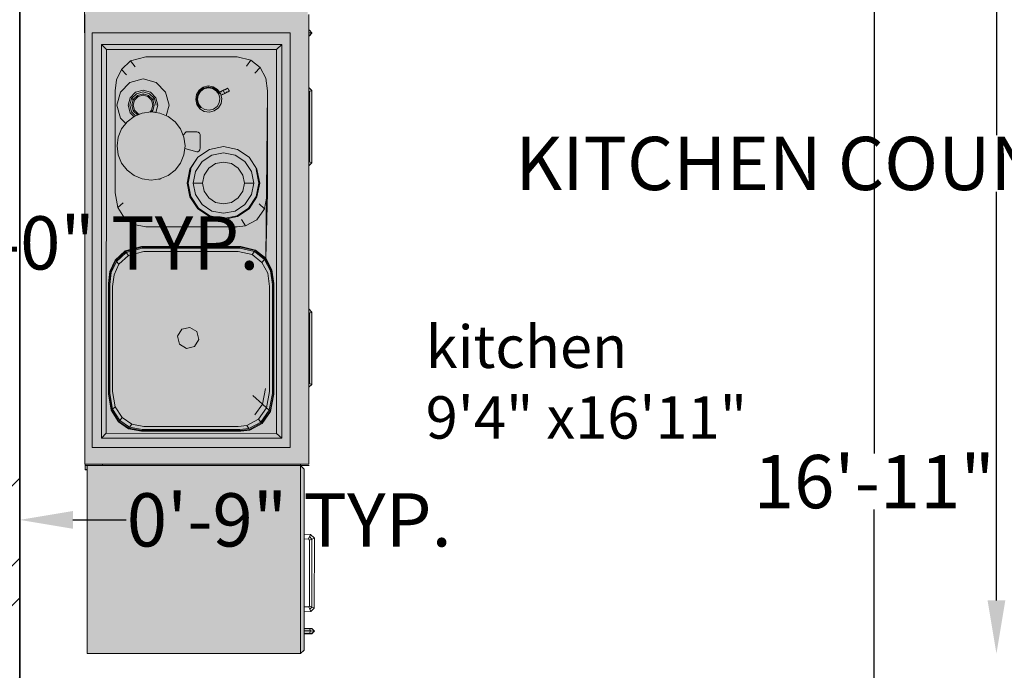
# Model space of a CAD drawing. Units: inches. Extents: x 3614 to 4242, y 2406 to 3033.
# Tile 4 of 10: x 3697 to 3808, y 2823 to 2896. Entities that reach past the tile are written whole.
import ezdxf

# ---------------------------------------------------------------- set-up
doc = ezdxf.new("R2010")
doc.units = ezdxf.units.IN
for name, color, linetype, lineweight in [('A-ANNO-DIMS', 2, 'Continuous', 18), ('A-AREA-IDEN', 7, 'Continuous', 25), ('A-FLOR-FIXT', 9, 'Continuous', 18), ('A-WALL', 7, 'Continuous', 35), ('A-WALL-PATT', 252, 'Continuous', 13)]:
    doc.layers.add(name, color=color, linetype=linetype, lineweight=lineweight)
doc.layers.add('hatch', color=254, linetype='Continuous')
doc.styles.get("Standard").update_dxf_attribs({"font": 'arial.ttf'})
doc.dimstyles.get("Standard").update_dxf_attribs({"dimtxt": 6, "dimasz": 6, "dimexe": 0.18, "dimexo": 0.0625, "dimgap": 0.09, "dimtad": 0, "dimtih": 1, "dimtoh": 1, "dimdec": 4, "dimzin": 0, "dimdsep": 46, "dimlunit": 4, "dimtxsty": 'Standard', "dimcen": 0.09, "dimse1": 1, "dimse2": 1, "dimadec": 0, "dimazin": 0, "dimtfac": 1, "dimtdec": 4, "dimtofl": 0, "dimtmove": 0, "dimatfit": 3, "dimfxl": 1, "dimtolj": 1, "dimtzin": 0, "dimarcsym": 0})

# ---------------------------------------------------------------- blocks, each defined once
blk = doc.blocks.new('kithen1')
at = {"layer": 'hatch'}
blk.add_hatch(color=256, dxfattribs=at).paths.add_polyline_path([(-2799.7, -8.3), (-2273.3, -8.3), (-2273.3, -1.7), (-2257.5, -1.7), (-2257.5, -1.1), (-1023.7, -1.1), (-1023.7, 0), (0, 0), (0, -0.3), (0.3, -0.3), (0.3, -1009.9), (-6.1, -1009.9), (-6.1, -2189.3), (-615.8, -2189.3), (-626.5, -2178.9), (-626.5, -1578.2), (-615.8, -1567.8), (-649.5, -1567.8), (-649.5, -1399.1), (-650.3, -1399.1), (-650.3, -1376.8), (-657.9, -1368.5), (-657.8, -1162.4), (-650.3, -1155.1), (-650.3, -1126.4), (-649.5, -1126.4), (-649.5, -1081.1), (-650.3, -1081.1), (-650.3, -1021.1), (-649.5, -1021.1), (-649.5, -959.1), (-651, -959.1), (-650.7, -903), (-653.5, -903), (-660.6, -895.5), (-660.5, -894.6), (-653.5, -887.1), (-651, -887.1), (-651, -638.7), (-651.2, -638.5), (-898.3, -638.5), (-898.3, -640.4), (-905.9, -647.4), (-906.8, -647.4), (-914.3, -640.4), (-914.3, -638.5), (-971.4, -638.5), (-971.4, -642.6), (-1016.2, -642.6), (-1016.2, -643.9), (-1023.8, -650.9), (-1024.7, -650.9), (-1032.2, -643.9), (-1032.2, -642.6), (-1179.7, -642.6), (-1188.8, -650.9), (-1395.6, -650.9), (-1403.7, -642.6), (-1813.5, -642.6), (-1822.6, -650.9), (-2029.4, -650.9), (-2037.5, -642.6), (-2257.5, -642.6), (-2257.5, -618.1), (-2261.3, -618.1), (-2271.7, -628.7), (-2458, -628.7), (-2727.7, -628.7), (-2727.7, -651.1), (-2735, -658.1), (-2735.9, -658), (-2743.2, -651.1), (-2743.2, -628.7), (-2789.4, -628.7), (-2799.7, -618.1)])
at = {"color": 0}
for p, q in [((0, 0), (-1023.7, 0)), ((-2261.3, -8.3), (-2799.7, -8.3)), ((-2799.7, -8.3), (-2799.7, -618.1)), ((-2273.3, -1.9), (-2273.9, -1.9)), ((-2273.9, -1.9), (-2273.9, -8.3)), ((-2261.3, -1.7), (-2273.3, -1.7)), ((-2273.3, -1.7), (-2273.3, -8.3)), ((-2261.3, -601.6), (-2261.3, -1.7)), ((-2261.3, -618.1), (-2261.3, -8.3)), ((-2261, -8.5), (-2261.3, -8.5)), ((-971.4, -1.1), (-2257.5, -1.1)), ((-2257.5, -1.1), (-2257.5, -642.6)), ((-1023.7, -22.5), (-2210.1, -22.5)), ((-2210.1, -22.5), (-2210.1, -589.1)), ((-1023.7, -589.1), (-1023.7, -22.5)), ((-2257.5, -51.5), (-2261.3, -51.5)), ((-2261.3, -51.5), (-2261.3, -536.3)), ((-2183.7, -48.8), (-1056.9, -48.9)), ((-2169.4, -62.7), (-2183.7, -48.8)), ((-2183.7, -48.8), (-2183.7, -565)), ((-1056.9, -48.9), (-1071, -63.6)), ((-1056.9, -48.9), (-1056.9, -565)), ((-2169.7, -550.2), (-2169.4, -62.7)), ((-1071, -63.6), (-2169.4, -62.7)), ((-2103.6, -76.6), (-2136.6, -97.6)), ((-2135.1, -98.9), (-2102.3, -78.1)), ((-2100.1, -80.6), (-2132.5, -101.2)), ((-2057.7, -68.5), (-2103.6, -76.6)), ((-2102.3, -78.1), (-2056.8, -70)), ((-2100.1, -80.6), (-2102.3, -78.1)), ((-2055, -72.6), (-2100.1, -80.6)), ((-2093.2, -88.3), (-2100.1, -80.6)), ((-2049.7, -80.6), (-2093.2, -88.3)), ((-1740.9, -68.5), (-2057.7, -68.5)), ((-2056.8, -70), (-1741.9, -70)), ((-1743.7, -72.6), (-2055, -72.6)), ((-1749, -80.6), (-2049.7, -80.6)), ((-1716.2, -84.8), (-1749, -80.6)), ((-1709.7, -76.9), (-1743.7, -72.6)), ((-1741.9, -70), (-1707.6, -74.4)), ((-1706.4, -72.9), (-1740.9, -68.5)), ((-1678, -91.5), (-1709.7, -76.9)), ((-1707.6, -74.4), (-1675.5, -89.1)), ((-1674.1, -87.7), (-1706.4, -72.9)), ((-1071, -550.2), (-1071, -63.6)), ((-2136.6, -97.6), (-2156.1, -126.2)), ((-2154.5, -127.3), (-2135.1, -98.9)), ((-2132.5, -101.2), (-2151.7, -129.3)), ((-2124.5, -108.2), (-2143, -135.3)), ((-2132.5, -101.2), (-2135.1, -98.9)), ((-2124.5, -108.2), (-2132.5, -101.2)), ((-2093.2, -88.3), (-2124.5, -108.2)), ((-1685.6, -98.8), (-1716.2, -84.8)), ((-1678, -91.5), (-1685.6, -98.8)), ((-1685.6, -98.8), (-1660.4, -125.8)), ((-1651.9, -119.5), (-1678, -91.5)), ((-1675.5, -89.1), (-1649.1, -117.4)), ((-1647.6, -116.2), (-1674.1, -87.7)), ((-1523.7, -95.6), (-1554, -114.9)), ((-1481.5, -88.1), (-1523.7, -95.6)), ((-1523.7, -95.6), (-1509.8, -111.1)), ((-1189.8, -88.1), (-1481.5, -88.1)), ((-1416.2, -122.1), (-1396, -106.6)), ((-1396, -106.6), (-1372.5, -96.9)), ((-1372.5, -96.9), (-1347.3, -93.6)), ((-1347.3, -93.6), (-1322, -96.9)), ((-1322, -96.9), (-1298.5, -106.6)), ((-1298.5, -106.6), (-1278.3, -122.1)), ((-1283.4, -118.2), (-1268.1, -102.9)), ((-1268.1, -102.9), (-1230.5, -92.9)), ((-1230.5, -92.9), (-1193, -102.9)), ((-1193, -102.9), (-1165.5, -130.3)), ((-1157.9, -92.2), (-1189.8, -88.1)), ((-1128.2, -105.8), (-1157.9, -92.2)), ((-1143.5, -120.5), (-1128.2, -105.8)), ((-1128.2, -105.8), (-1103.8, -132)), ((-2156.1, -126.2), (-2163.3, -163.2)), ((-2161.7, -164.1), (-2154.5, -127.3)), ((-2151.7, -129.3), (-2158.8, -165.7)), ((-2151.7, -129.3), (-2154.5, -127.3)), ((-2143, -135.3), (-2151.7, -129.3)), ((-2149.9, -170.5), (-2143, -135.3)), ((-1660.4, -125.8), (-1651.9, -119.5)), ((-1648.8, -170.4), (-1660.4, -125.8)), ((-1649.1, -117.4), (-1651.9, -119.5)), ((-1651.9, -119.5), (-1639.9, -165.7)), ((-1649.1, -117.4), (-1637, -164.1)), ((-1635.3, -163.2), (-1647.6, -116.2)), ((-1554, -114.9), (-1572, -141.2)), ((-1431.7, -142.2), (-1416.2, -122.1)), ((-1278.3, -122.1), (-1262.8, -142.2)), ((-1252, -130.7), (-1263.1, -141.8)), ((-1249.5, -134.9), (-1261, -146.4)), ((-1246.6, -139.9), (-1258.4, -151.7)), ((-1252, -130.7), (-1230.5, -124.9)), ((-1249.5, -134.9), (-1230.5, -129.8)), ((-1230.5, -135.6), (-1246.6, -139.9)), ((-1246.6, -139.9), (-1244.8, -143)), ((-1244.8, -143), (-1230.5, -139.2)), ((-1230.5, -124.9), (-1209.1, -130.7)), ((-1230.5, -129.8), (-1211.6, -134.9)), ((-1214.5, -139.9), (-1230.5, -135.6)), ((-1230.5, -135.6), (-1230.5, -139.2)), ((-1230.5, -139.2), (-1216.3, -143)), ((-1216.3, -143), (-1214.5, -139.9)), ((-1211.6, -134.9), (-1214.5, -139.9)), ((-1214.5, -139.9), (-1202.7, -151.7)), ((-1211.6, -134.9), (-1197.7, -148.8)), ((-1209.1, -130.7), (-1193.4, -146.3)), ((-1165.5, -130.3), (-1155.5, -167.7)), ((-1103.8, -132), (-1120.8, -144.8)), ((-1103.8, -132), (-1092.5, -175.3)), ((-2163.3, -163.2), (-2163.3, -447.5)), ((-2161.7, -446.6), (-2161.7, -164.1)), ((-2158.8, -165.7), (-2158.8, -445)), ((-1639.9, -165.7), (-1639.9, -445)), ((-1637, -164.1), (-1637, -446.6)), ((-1635.3, -447.4), (-1635.3, -163.2)), ((-1572, -141.2), (-1578.6, -175.3)), ((-1572, -141.2), (-1554.6, -153.3)), ((-1444.8, -190.8), (-1441.5, -165.7)), ((-1441.5, -165.7), (-1431.7, -142.2)), ((-1262.8, -142.2), (-1253, -165.7)), ((-1258.4, -151.7), (-1258.6, -152.3)), ((-1255.2, -153.5), (-1258.4, -151.7)), ((-1255.2, -153.5), (-1256.4, -157.6)), ((-1244.8, -143), (-1255.2, -153.5)), ((-1253, -165.7), (-1249.7, -190.8)), ((-1205.8, -153.5), (-1216.3, -143)), ((-1202.7, -151.7), (-1205.8, -153.5)), ((-1205.8, -153.5), (-1202, -167.7)), ((-1202, -167.7), (-1205.8, -181.9)), ((-1198.4, -167.7), (-1202.7, -151.7)), ((-1202.7, -183.7), (-1198.4, -167.7)), ((-1202, -167.7), (-1198.4, -167.7)), ((-1197.7, -148.8), (-1192.6, -167.7)), ((-1192.6, -167.7), (-1197.7, -186.6)), ((-1193.4, -146.3), (-1187.6, -167.7)), ((-1187.6, -167.7), (-1193.4, -189.1)), ((-1155.5, -167.7), (-1165.5, -205.1)), ((-2149.9, -440.2), (-2149.9, -170.5)), ((-1648.8, -440.2), (-1648.8, -170.4)), ((-1578.6, -175.3), (-1578.6, -437)), ((-1441.5, -216), (-1444.8, -190.8)), ((-1249.7, -190.8), (-1253, -216)), ((-1250.2, -186.9), (-1244.8, -192.3)), ((-1246.6, -195.5), (-1249.9, -192.2)), ((-1244.8, -192.3), (-1246.6, -195.5)), ((-1230.5, -199.7), (-1246.6, -195.5)), ((-1230.5, -196.1), (-1244.8, -192.3)), ((-1216.3, -192.3), (-1230.5, -196.1)), ((-1214.5, -195.5), (-1230.5, -199.7)), ((-1230.5, -196.1), (-1230.5, -199.7)), ((-1205.8, -181.9), (-1216.3, -192.3)), ((-1216.3, -192.3), (-1214.5, -195.5)), ((-1214.5, -195.5), (-1202.7, -183.7)), ((-1211.6, -200.5), (-1214.5, -195.5)), ((-1197.7, -186.6), (-1211.6, -200.5)), ((-1193.4, -189.1), (-1209.1, -204.7)), ((-1205.8, -181.9), (-1202.7, -183.7)), ((-1092.5, -175.3), (-1092.5, -437)), ((-1442, -212), (-1442.1, -213.6)), ((-1442.1, -213.6), (-1441.9, -216.3)), ((-1441.9, -216.3), (-1441.5, -218.2)), ((-1431.7, -239.4), (-1441.5, -216)), ((-1441.5, -218.2), (-1440.8, -218.9)), ((-1440.8, -218.9), (-1440.3, -218.9)), ((-1253, -216), (-1262.8, -239.4)), ((-1230.5, -210.4), (-1251.6, -204.8)), ((-1250.8, -199.1), (-1249.5, -200.5)), ((-1211.6, -200.5), (-1230.5, -205.5)), ((-1209.1, -204.7), (-1230.5, -210.4)), ((-1165.5, -205.1), (-1193, -232.5)), ((-1416.2, -259.6), (-1431.7, -239.4)), ((-1262.8, -239.4), (-1278.3, -259.6)), ((-1230.5, -242.5), (-1260.7, -234.4)), ((-1193, -232.5), (-1230.5, -242.5)), ((-1914.6, -272.1), (-1926.9, -292)), ((-1891.8, -266.6), (-1914.6, -272.1)), ((-1871.8, -278.8), (-1891.8, -266.6)), ((-1866.3, -301.6), (-1871.8, -278.8)), ((-1396, -275), (-1416.2, -259.6)), ((-1372.5, -284.8), (-1396, -275)), ((-1298.5, -275), (-1322, -284.8)), ((-1278.3, -259.6), (-1298.5, -275)), ((-1926.9, -292), (-1921.4, -314.8)), ((-1878.5, -321.5), (-1866.3, -301.6)), ((-1526.8, -324.6), (-1493.1, -302.1)), ((-1493.1, -302.2), (-1526.8, -324.6)), ((-1492.2, -304.2), (-1525.2, -326.2)), ((-1493.1, -302.1), (-1453.2, -294.2)), ((-1453.2, -294.3), (-1493.1, -302.2)), ((-1453.2, -296.5), (-1492.2, -304.2)), ((-1453.2, -294.2), (-1413.4, -302.1)), ((-1413.4, -302.2), (-1453.2, -294.3)), ((-1453.2, -294.3), (-1453.2, -296.5)), ((-1453.2, -296.5), (-1414.2, -304.2)), ((-1413.4, -302.1), (-1379.6, -324.6)), ((-1379.6, -324.6), (-1413.4, -302.2)), ((-1347.3, -288.1), (-1372.5, -284.8)), ((-1364, -321.4), (-1354.5, -287.1)), ((-1322, -284.8), (-1347.3, -288.1)), ((-1316.5, -282.5), (-1307.2, -290.8)), ((-1307.2, -290.8), (-1307.2, -321.4)), ((-1921.4, -314.8), (-1901.4, -327)), ((-1901.4, -327), (-1878.5, -321.5)), ((-1526.8, -324.6), (-1549.4, -358.3)), ((-1549.4, -358.3), (-1526.8, -324.6)), ((-1525.2, -326.2), (-1547.3, -359.2)), ((-1514.5, -337), (-1533.3, -365)), ((-1486.4, -318.2), (-1514.5, -337)), ((-1453.2, -311.7), (-1486.4, -318.2)), ((-1453.2, -311.7), (-1420.1, -318.2)), ((-1453.2, -338.2), (-1453.2, -311.7)), ((-1420.1, -318.2), (-1392, -337)), ((-1392, -337), (-1373.2, -365)), ((-1379.6, -324.6), (-1357, -358.3)), ((-1357, -358.3), (-1379.6, -324.6)), ((-1363.6, -324.3), (-1364, -321.4)), ((-1361.6, -328), (-1363.6, -324.3)), ((-1357.9, -330.6), (-1361.6, -328)), ((-1352.7, -331.6), (-1357.9, -330.6)), ((-1318.5, -331.6), (-1352.7, -331.6)), ((-1314.3, -331), (-1318.5, -331.6)), ((-1310.7, -329.1), (-1314.3, -331)), ((-1308.2, -326), (-1310.7, -329.1)), ((-1307.2, -321.4), (-1308.2, -326)), ((-1248.3, -343.1), (-1240.7, -330.6)), ((-1243.2, -344.9), (-1236.8, -334.2)), ((-1240.7, -330.6), (-1228.9, -321.9)), ((-1227.6, -324.8), (-1238.3, -332.8)), ((-1236.8, -334.2), (-1226.7, -326.8)), ((-1228.9, -321.9), (-1214.7, -318.4)), ((-1227.6, -324.8), (-1228.3, -323.3)), ((-1214.6, -321.6), (-1227.6, -324.8)), ((-1226.7, -326.8), (-1214.5, -323.7)), ((-1214.7, -318.4), (-1200.3, -320.6)), ((-1214.7, -319.9), (-1214.6, -321.6)), ((-1214.6, -321.6), (-1201.4, -323.6)), ((-1214.5, -323.7), (-1202.1, -325.6)), ((-1202.1, -325.6), (-1191.3, -332)), ((-1201.4, -323.6), (-1200.8, -322)), ((-1201.4, -323.6), (-1189.9, -330.5)), ((-1200.3, -320.6), (-1187.7, -328.1)), ((-1191.3, -332), (-1183.9, -342.1)), ((-1189.9, -330.5), (-1188.7, -329.2)), ((-1189.9, -330.5), (-1181.9, -341.2)), ((-1187.7, -328.1), (-1179, -339.8)), ((-1549.4, -358.3), (-1557.3, -398)), ((-1557.3, -398), (-1549.4, -358.3)), ((-1547.3, -359.2), (-1555.1, -398)), ((-1533.3, -365), (-1539.9, -398)), ((-1508.7, -375.1), (-1495.7, -355.7)), ((-1495.7, -355.7), (-1476.2, -342.8)), ((-1476.2, -342.8), (-1453.2, -338.2)), ((-1430.3, -342.8), (-1453.2, -338.2)), ((-1410.8, -355.7), (-1430.3, -342.8)), ((-1397.8, -375.1), (-1410.8, -355.7)), ((-1373.2, -365), (-1366.6, -398)), ((-1357, -358.3), (-1349.1, -398)), ((-1349.1, -398), (-1357, -358.3)), ((-1250.4, -357.6), (-1248.3, -343.1)), ((-1246.9, -371.7), (-1250.4, -357.6)), ((-1245.1, -357.3), (-1243.2, -344.9)), ((-1242, -369.4), (-1245.1, -357.3)), ((-1183.9, -342.1), (-1180.8, -354.2)), ((-1180.8, -354.2), (-1182.7, -366.6)), ((-1181.9, -341.2), (-1180.4, -340.5)), ((-1181.9, -341.2), (-1178.7, -354.1)), ((-1178.7, -354.1), (-1180.7, -367.3)), ((-1179, -339.8), (-1175.5, -354)), ((-1178.7, -354.1), (-1177, -354.1)), ((-1175.5, -354), (-1177.6, -368.4)), ((-1513.2, -398), (-1508.7, -375.1)), ((-1393.2, -398), (-1397.8, -375.1)), ((-1238.2, -383.5), (-1246.9, -371.7)), ((-1234.6, -379.5), (-1242, -369.4)), ((-1225.6, -391), (-1238.2, -383.5)), ((-1223.8, -385.9), (-1234.6, -379.5)), ((-1211.2, -393.1), (-1225.6, -391)), ((-1211.4, -387.8), (-1223.8, -385.9)), ((-1199.2, -384.8), (-1211.4, -387.8)), ((-1197, -389.6), (-1211.2, -393.1)), ((-1202.1, -390.9), (-1202.4, -391)), ((-1202.4, -391), (-1202, -390.9)), ((-1202.4, -391), (-1202.4, -391)), ((-1202.4, -391), (-1202.3, -391.3)), ((-1202.3, -391.3), (-1200.2, -395.7)), ((-1202, -390.9), (-1202.1, -390.9)), ((-1201.7, -390.8), (-1199.7, -395.1)), ((-1199.7, -395.1), (-1198, -394.1)), ((-1189.2, -377.3), (-1199.2, -384.8)), ((-1187.6, -378.8), (-1198.3, -386.7)), ((-1185.2, -380.9), (-1197, -389.6)), ((-1193.3, -386.9), (-1194.2, -387.6)), ((-1193.1, -386.7), (-1193.3, -386.9)), ((-1193.3, -386.9), (-1191.3, -391.2)), ((-1191.3, -391.2), (-1193.2, -391.8)), ((-1192.7, -386.5), (-1192.9, -386.6)), ((-1192.6, -386.8), (-1192.7, -386.5)), ((-1190.5, -391.2), (-1192.6, -386.8)), ((-1191.3, -391.2), (-1190.5, -391.2)), ((-1188.3, -397.5), (-1191.3, -391.2)), ((-1190.5, -391.2), (-1187.6, -397.2)), ((-1182.7, -366.6), (-1189.2, -377.3)), ((-1180.7, -367.3), (-1187.6, -378.8)), ((-1187.6, -378.8), (-1186.3, -379.9)), ((-1177.6, -368.4), (-1185.2, -380.9)), ((-1180.7, -367.3), (-1179.1, -367.9)), ((-1557.3, -398), (-1549.4, -437.8)), ((-1549.4, -437.8), (-1557.3, -398)), ((-1555.1, -398), (-1547.3, -436.9)), ((-1539.9, -398), (-1533.3, -431.1)), ((-1508.7, -420.9), (-1513.2, -398)), ((-1495.7, -440.4), (-1508.7, -420.9)), ((-1410.8, -440.4), (-1397.8, -420.9)), ((-1397.8, -420.9), (-1393.2, -398)), ((-1366.6, -398), (-1373.2, -431.1)), ((-1349.1, -398), (-1357, -437.8)), ((-1357, -437.8), (-1349.1, -398)), ((-1200.2, -395.7), (-1199.7, -395.1)), ((-1200.2, -395.7), (-1197.3, -401.8)), ((-1199.7, -395.1), (-1196.7, -401.5)), ((-1197.3, -401.8), (-1196.7, -401.5)), ((-1197.3, -401.8), (-1194.5, -407.8)), ((-1196.7, -401.5), (-1190.1, -398.4)), ((-1196.7, -401.5), (-1193.7, -407.8)), ((-1194.5, -407.8), (-1193.7, -407.8)), ((-1192.4, -412.2), (-1194.5, -407.8)), ((-1193.7, -407.8), (-1191.8, -407.2)), ((-1193.7, -407.8), (-1191.5, -412.5)), ((-1191.6, -413.9), (-1192.4, -412.2)), ((-1190.7, -414.2), (-1191.6, -413.9)), ((-1188.7, -413.8), (-1190.7, -414.2)), ((-1190.1, -398.4), (-1188.3, -397.5)), ((-1186.2, -412.8), (-1188.7, -413.8)), ((-1187.6, -397.2), (-1188.3, -397.5)), ((-1188.3, -397.5), (-1185.3, -403.9)), ((-1184.8, -403.3), (-1187.6, -397.2)), ((-1185.3, -403.9), (-1186.9, -404.9)), ((-1183.8, -411.5), (-1186.2, -412.8)), ((-1185.3, -403.9), (-1184.8, -403.3)), ((-1183.1, -408.5), (-1185.3, -403.9)), ((-1184.8, -403.3), (-1182.7, -407.7)), ((-1182.3, -410.2), (-1183.8, -411.5)), ((-1182.7, -407.7), (-1181.9, -409.3)), ((-1181.9, -409.3), (-1182.3, -410.2)), ((-2163.3, -447.5), (-2159.9, -473.6)), ((-2158.2, -472.6), (-2161.7, -446.6)), ((-2158.8, -445), (-2155.4, -470.7)), ((-2146.6, -465), (-2149.9, -440.2)), ((-1658, -480.4), (-1648.8, -440.2)), ((-1639.9, -445), (-1649.4, -486.6)), ((-1637, -446.6), (-1646.6, -488.6)), ((-1645, -489.8), (-1635.3, -447.4)), ((-1578.6, -437), (-1575.5, -461.1)), ((-1575.5, -461.1), (-1557.8, -449.7)), ((-1549.4, -437.8), (-1526.8, -471.4)), ((-1526.8, -471.4), (-1549.4, -437.8)), ((-1547.3, -436.9), (-1525.2, -469.8)), ((-1533.3, -431.1), (-1514.5, -459.1)), ((-1476.2, -453.3), (-1495.7, -440.4)), ((-1430.3, -453.3), (-1410.8, -440.4)), ((-1373.2, -431.1), (-1392, -459.1)), ((-1357, -437.8), (-1379.6, -471.4)), ((-1379.6, -471.4), (-1357, -437.8)), ((-1092.5, -437), (-1101.4, -476)), ((-2159.9, -473.6), (-2141.1, -508.3)), ((-2139.6, -507.1), (-2158.2, -472.6)), ((-2155.4, -470.7), (-2146.6, -465)), ((-2137, -504.8), (-2155.4, -470.7)), ((-2146.6, -465), (-2128.8, -498)), ((-1575.5, -461.1), (-1558.2, -493)), ((-1493.1, -493.9), (-1526.8, -471.4)), ((-1526.8, -471.4), (-1493.1, -493.9)), ((-1525.2, -469.8), (-1492.2, -491.9)), ((-1514.5, -459.1), (-1486.4, -477.9)), ((-1486.4, -477.9), (-1453.2, -484.4)), ((-1453.2, -457.9), (-1476.2, -453.3)), ((-1453.2, -457.9), (-1430.3, -453.3)), ((-1453.2, -484.4), (-1453.2, -457.9)), ((-1420.1, -477.9), (-1453.2, -484.4)), ((-1392, -459.1), (-1420.1, -477.9)), ((-1379.6, -471.4), (-1413.4, -493.9)), ((-1413.4, -493.9), (-1379.6, -471.4)), ((-1101.4, -476), (-1123, -502.7)), ((-1101.4, -476), (-1118.7, -463.5)), ((-2137, -504.8), (-2139.6, -507.1)), ((-2105.6, -531.3), (-2139.6, -507.1)), ((-2128.8, -498), (-2137, -504.8)), ((-2103.3, -528.8), (-2137, -504.8)), ((-2128.8, -498), (-2096.3, -521.1)), ((-2085.5, -509.3), (-2116.3, -487.4)), ((-2060.9, -482.3), (-2085.5, -509.3)), ((-1680.2, -507.9), (-1658, -480.4)), ((-1649.4, -486.6), (-1672.5, -515.1)), ((-1646.6, -488.6), (-1669.9, -517.4)), ((-1668.5, -518.8), (-1645, -489.8)), ((-1649.4, -486.6), (-1658, -480.4)), ((-1646.6, -488.6), (-1649.4, -486.6)), ((-1558.2, -493), (-1526.7, -515.5)), ((-1526.7, -515.5), (-1512.6, -500.1)), ((-1453.2, -501.8), (-1493.1, -493.9)), ((-1493.1, -493.9), (-1453.2, -501.8)), ((-1492.2, -491.9), (-1453.2, -499.6)), ((-1453.2, -499.6), (-1414.2, -491.9)), ((-1413.4, -493.9), (-1453.2, -501.8)), ((-1453.2, -501.8), (-1413.4, -493.9)), ((-1453.2, -499.6), (-1453.2, -501.8)), ((-1123, -502.7), (-1153.4, -518.8)), ((-1123, -502.7), (-1138.7, -488.2)), ((-2257.5, -535.3), (-2257.9, -535.3)), ((-2141.1, -508.3), (-2106.9, -532.7)), ((-2106.9, -532.7), (-2057.7, -542.2)), ((-2103.3, -528.8), (-2105.6, -531.3)), ((-2056.8, -540.7), (-2105.6, -531.3)), ((-2096.3, -521.1), (-2103.3, -528.8)), ((-2055, -538.1), (-2103.3, -528.8)), ((-2096.3, -521.1), (-2085.5, -509.3)), ((-2049.7, -530.1), (-2096.3, -521.1)), ((-2085.5, -509.3), (-2041.5, -517.8)), ((-1749, -530.1), (-2049.7, -530.1)), ((-1749, -530.1), (-1797.1, -530.1)), ((-1711.5, -524.5), (-1749, -530.1)), ((-1704.9, -532.3), (-1743.7, -538.1)), ((-1741.9, -540.7), (-1702.7, -534.9)), ((-1680.2, -507.9), (-1711.5, -524.5)), ((-1672.5, -515.1), (-1704.9, -532.3)), ((-1702.7, -534.9), (-1669.9, -517.4)), ((-1668.5, -518.8), (-1701.5, -536.3)), ((-1672.5, -515.1), (-1680.2, -507.9)), ((-1669.9, -517.4), (-1672.5, -515.1)), ((-1189.8, -524.2), (-1668.5, -518.8)), ((-1481.5, -524.2), (-1668.5, -518.8)), ((-1526.7, -515.5), (-1481.5, -524.2)), ((-1189.8, -524.2), (-1481.5, -524.2)), ((-1153.4, -518.8), (-1189.8, -524.2)), ((-2183.7, -565), (-2169.7, -550.2)), ((-1793.1, -550.2), (-2169.7, -550.2)), ((-2057.7, -542.2), (-2056.8, -540.7)), ((-1783.5, -542.2), (-2057.7, -542.2)), ((-1781.7, -540.7), (-2056.8, -540.7)), ((-1778.6, -538.1), (-2055, -538.1)), ((-1743.7, -538.1), (-1797.1, -538.1)), ((-1741.9, -540.7), (-1797.1, -540.7)), ((-1740.9, -542.2), (-1797.1, -542.2)), ((-1071, -550.2), (-1797.1, -550.2)), ((-1740.9, -542.2), (-1741.9, -540.7)), ((-1701.5, -536.3), (-1740.9, -542.2)), ((-1056.9, -565), (-1071, -550.2)), ((-2210.1, -589.1), (-1789.4, -589.1)), ((-1797.1, -565), (-2183.7, -565)), ((-1056.9, -565), (-1797.1, -565)), ((-1797.1, -589.1), (-1023.7, -589.1)), ((-2799.7, -618.1), (-2261.3, -618.1)), ((-2789.4, -628.7), (-2799.7, -618.1)), ((-2261.3, -618.1), (-2271.7, -628.7)), ((-2261, -596.4), (-2261.3, -596.4)), ((-2261.3, -626.3), (-2261.3, -601.6)), ((-2271.7, -628.7), (-2789.4, -628.7)), ((-2743.2, -628.7), (-2743.2, -644.8)), ((-2743.2, -644.8), (-2742.3, -644.5)), ((-2743.2, -651.1), (-2743.2, -644.8)), ((-2742.3, -628.7), (-2742.3, -644.4)), ((-2742.3, -644.4), (-2734.9, -647.4)), ((-2742.3, -644.4), (-2742.3, -651.1)), ((-2734.9, -647.4), (-2735, -658.1)), ((-2734.9, -647.4), (-2734.9, -628.7)), ((-2727.7, -644.4), (-2734.9, -647.4)), ((-2727.7, -628.7), (-2727.7, -644.4)), ((-2727.7, -651.1), (-2727.7, -644.4)), ((-2679.7, -628.7), (-2679.4, -647.7)), ((-2679.4, -647.7), (-2665.9, -642)), ((-2669.5, -658), (-2679.4, -647.7)), ((-2666.7, -651.1), (-2672.6, -644.8)), ((-2663.9, -644.2), (-2666.7, -651.1)), ((-2665.6, -628.7), (-2665.9, -642)), ((-2665.9, -642), (-2663.9, -644.2)), ((-2663.9, -644.2), (-2474.9, -644.1)), ((-2474.9, -644.1), (-2471.7, -641.3)), ((-2474.9, -644.1), (-2472.3, -651.1)), ((-2472.3, -651.1), (-2465, -644.4)), ((-2471.7, -641.3), (-2472, -628.7)), ((-2458.4, -647.4), (-2471.7, -641.3)), ((-2458.4, -647.4), (-2469.7, -658.1)), ((-2458, -628.7), (-2458.4, -647.4)), ((-2261.3, -643.6), (-2261.3, -626.3)), ((-2257.5, -642.6), (-1797.1, -642.6)), ((-2037.5, -642.6), (-2029.4, -650.9)), ((-2029.4, -650.9), (-2026.5, -643.9)), ((-2026.5, -643.9), (-2027.8, -642.6)), ((-2025.9, -642.6), (-2026.5, -643.9)), ((-2026.5, -643.9), (-1828.9, -643.9)), ((-1825.3, -643.9), (-1828.9, -643.9)), ((-1825.8, -642.6), (-1825.3, -643.9)), ((-1825.3, -643.9), (-1823.8, -642.6)), ((-1822.6, -650.9), (-1825.3, -643.9)), ((-1813.5, -642.6), (-1822.6, -650.9)), ((-971.4, -642.6), (-1797.1, -642.6)), ((-1395.6, -650.9), (-1403.7, -642.6)), ((-1392.7, -643.9), (-1395.6, -650.9)), ((-1394, -642.6), (-1392.7, -643.9)), ((-1392.7, -643.9), (-1392.1, -642.6)), ((-1191.5, -643.9), (-1392.7, -643.9)), ((-1192, -642.6), (-1191.5, -643.9)), ((-1191.5, -643.9), (-1190, -642.6)), ((-1188.8, -650.9), (-1191.5, -643.9)), ((-1179.7, -642.6), (-1188.8, -650.9)), ((-1032.2, -643.9), (-1032.2, -642.6)), ((-1031.4, -643.1), (-1032.2, -643.9)), ((-1031.4, -643.9), (-1032.2, -643.9)), ((-1032.2, -643.9), (-1024.7, -650.9)), ((-1031.4, -642.6), (-1031.4, -643.9)), ((-1023.8, -650.9), (-1031.4, -643.9)), ((-1023.8, -650.9), (-1023.8, -642.6)), ((-1016.2, -643.9), (-1023.8, -650.9)), ((-1016.2, -642.6), (-1016.2, -643.9)), ((-2742.3, -650.3), (-2743.2, -651.1)), ((-2742.3, -651.1), (-2743.2, -651.1)), ((-2743.2, -651.1), (-2735.9, -658)), ((-2735, -658.1), (-2742.3, -651.1)), ((-2735.9, -658), (-2735, -658.1)), ((-2735, -658.1), (-2727.7, -651.1)), ((-2666.7, -651.1), (-2669.5, -658)), ((-2669.5, -658), (-2469.7, -658.1)), ((-2472.3, -651.1), (-2666.7, -651.1)), ((-2469.7, -658.1), (-2472.3, -651.1)), ((-2029.4, -650.9), (-1828.9, -650.9)), ((-1822.6, -650.9), (-1828.9, -650.9)), ((-1395.6, -650.9), (-1188.8, -650.9)), ((-1024.7, -650.9), (-1023.8, -650.9))]:
    blk.add_line(p, q, dxfattribs=at)
for points in [[(-2799.7, -8.3), (-2273.3, -8.3), (-2273.3, -1.7), (-2257.5, -1.7), (-2257.5, -1.1), (-1023.7, -1.1), (-1023.7, 0), (0, 0)], [(-971.4, -642.6), (-1016.2, -642.6), (-1016.2, -643.9), (-1023.8, -650.9), (-1024.7, -650.9), (-1032.2, -643.9), (-1032.2, -642.6), (-1179.7, -642.6), (-1188.8, -650.9), (-1395.6, -650.9), (-1403.7, -642.6), (-1813.5, -642.6), (-1822.6, -650.9), (-2029.4, -650.9), (-2037.5, -642.6), (-2257.5, -642.6), (-2257.5, -618.1), (-2261.3, -618.1), (-2271.7, -628.7), (-2458, -628.7), (-2727.7, -628.7), (-2727.7, -651.1), (-2735, -658.1), (-2735.9, -658), (-2743.2, -651.1), (-2743.2, -628.7), (-2789.4, -628.7), (-2799.7, -618.1), (-2799.7, -8.3)]]:
    blk.add_lwpolyline(points)
blk = doc.blocks.new('*D15')
at = {"layer": 'A-ANNO-DIMS', "color": 0, "lineweight": -2, "transparency": 16777216}
for p, q in [((3793.63, 2939.34), (3793.63, 2846.99)), ((3793.63, 2748.34), (3793.63, 2840.69))]:
    blk.add_line(p, q, dxfattribs=at)
at = {"layer": 'A-ANNO-DIMS', "color": 0, "transparency": 16777216}
for points in [[(3792.63, 2939.34), (3794.63, 2939.34), (3793.63, 2945.34)], [(3792.63, 2748.34), (3794.63, 2748.34), (3793.63, 2742.34)]]:
    blk.add_solid(points, dxfattribs=at)
at = {"layer": 'Defpoints', "color": 0, "transparency": 16777216}
for p in [(3799.84, 2945.34), (3793.63, 2742.34), (3799.84, 2742.34)]:
    blk.add_point(p, dxfattribs=at)
at = {"layer": 'A-ANNO-DIMS', "color": 0, "transparency": 16777216, "insert": (3793.63, 2843.84), "char_height": 6, "attachment_point": 5}
blk.add_mtext('\\A1;16\'-11"', dxfattribs=at)
blk = doc.blocks.new('*D41')
at = {"layer": 'A-ANNO-DIMS', "color": 0, "lineweight": -2, "transparency": 16777216}
for p, q in [((3681.14, 2888.73), (3681.14, 2873.93)), ((3681.14, 2852.73), (3681.14, 2867.54))]:
    blk.add_line(p, q, dxfattribs=at)
at = {"layer": 'A-ANNO-DIMS', "color": 0, "transparency": 16777216}
for points in [[(3680.14, 2888.73), (3682.14, 2888.73), (3681.14, 2894.73)], [(3680.14, 2852.73), (3682.14, 2852.73), (3681.14, 2846.73)]]:
    blk.add_solid(points, dxfattribs=at)
at = {"layer": 'Defpoints', "color": 0, "transparency": 16777216}
for p in [(3688.34, 2894.73), (3681.14, 2846.73), (3688.34, 2846.73)]:
    blk.add_point(p, dxfattribs=at)
at = {"layer": 'A-ANNO-DIMS', "color": 0, "transparency": 16777216, "insert": (3681.14, 2870.73), "char_height": 6, "attachment_point": 5}
blk.add_mtext('\\A1;WINDOW W1 4\'-0" TYP.', dxfattribs=at)
blk = doc.blocks.new('*D42')
at = {"layer": 'A-ANNO-DIMS', "color": 0, "lineweight": -2, "transparency": 16777216}
for p, q in [((3682.34, 2839.53), (3676.34, 2839.53)), ((3703.34, 2839.53), (3709.34, 2839.53))]:
    blk.add_line(p, q, dxfattribs=at)
at = {"layer": 'A-ANNO-DIMS', "color": 0, "transparency": 16777216}
for points in [[(3682.34, 2840.53), (3682.34, 2838.53), (3688.34, 2839.53)], [(3703.34, 2840.53), (3703.34, 2838.53), (3697.34, 2839.53)]]:
    blk.add_solid(points, dxfattribs=at)
at = {"layer": 'Defpoints', "color": 0, "transparency": 16777216}
for p in [(3688.34, 2846.73), (3697.34, 2846.73), (3697.34, 2839.53)]:
    blk.add_point(p, dxfattribs=at)
at = {"layer": 'A-ANNO-DIMS', "color": 0, "transparency": 16777216, "insert": (3727.71, 2839.53), "char_height": 6, "attachment_point": 5}
blk.add_mtext('\\A1;0\'-9" TYP.', dxfattribs=at)
blk = doc.blocks.new('*D63')
at = {"layer": 'A-ANNO-DIMS', "color": 0, "lineweight": -2, "transparency": 16777216}
for p, q in [((3807.39, 2928.9), (3807.39, 2882.88)), ((3807.39, 2830.46), (3807.39, 2876.49))]:
    blk.add_line(p, q, dxfattribs=at)
at = {"layer": 'A-ANNO-DIMS', "color": 0, "transparency": 16777216}
for points in [[(3806.39, 2928.9), (3808.39, 2928.9), (3807.39, 2934.9)], [(3806.39, 2830.46), (3808.39, 2830.46), (3807.39, 2824.46)]]:
    blk.add_solid(points, dxfattribs=at)
at = {"layer": 'Defpoints', "color": 0, "transparency": 16777216}
for p in [(3790.82, 2934.9), (3807.39, 2934.9), (3790.82, 2824.46)]:
    blk.add_point(p, dxfattribs=at)
at = {"layer": 'A-ANNO-DIMS', "color": 0, "transparency": 16777216, "insert": (3807.39, 2879.68), "char_height": 6, "attachment_point": 5}
blk.add_mtext('\\A1;KITCHEN COUNTER 9\'-2 1/2"', dxfattribs=at)

msp = doc.modelspace()

# ---------------------------------------------------------------- hatches: boundary and pattern name
at = {"layer": 'A-WALL-PATT'}
h = msp.add_hatch(dxfattribs=at)
h.set_pattern_fill('ANSI32', color=256)
h.paths.add_polyline_path([(4041.01458, 2954.34049), (3982.96188, 2954.34049), (3982.96188, 2945.34049), (3983.336, 2945.34049), (4041.01458, 2945.34049)])
h.paths.add_polyline_path([(3973.96188, 2954.34049), (3960.11861, 2954.34049), (3960.11861, 2945.34049), (3973.96188, 2945.34049)])
h.paths.add_polyline_path([(3936.11861, 2954.34049), (3901.17016, 2954.34049), (3901.17016, 2945.34049), (3913.336, 2945.34049), (3913.336, 2896.34049, -0.050382044), (3919.336, 2895.73437), (3919.336, 2945.34049), (3936.11861, 2945.34049)])
h.paths.add_polyline_path([(3983.336, 2945.34049), (3982.96188, 2945.34049), (3974.336, 2945.34049), (3974.336, 2873.34049), (3974.336, 2795.31105), (3983.336, 2795.31105), (3983.336, 2867.34049)])
h.paths.add_polyline_path([(3974.336, 2872.34049), (3919.336, 2872.34049), (3858.336, 2872.34049), (3858.336, 2866.34049), (3919.336, 2866.34049), (3974.336, 2866.34049)])
h.paths.add_polyline_path([(3877.17016, 2954.34049), (3852.34021, 2954.34049), (3852.34021, 2945.34049), (3852.336, 2896.34049), (3858.336, 2896.34049), (3858.336, 2945.34049), (3877.17016, 2945.34049)])
h.paths.add_polyline_path([(3871.94212, 2902.34049), (3858.336, 2902.34049), (3858.336, 2896.34049), (3871.336, 2896.34049, -0.050382044)], flags=0)
h.paths.add_polyline_path([(3913.336, 2902.34049), (3901.336, 2902.34049), (3901.336, 2896.34049), (3913.336, 2896.34049)], flags=17)
h.paths.add_polyline_path([(3858.336, 2872.34049), (3852.336, 2872.34049), (3852.336, 2866.34049), (3858.336, 2866.34049)])
h.paths.add_polyline_path([(3809.336, 2954.34049), (3764.4617, 2954.34049), (3764.4617, 2945.34049), (3809.336, 2945.34049)])
h.paths.add_polyline_path([(3716.4617, 2954.34049), (3697.336, 2954.34049), (3697.336, 2945.34049), (3716.4617, 2945.34049)])
h.paths.add_polyline_path([(3697.336, 2945.34049), (3688.336, 2945.34049), (3688.336, 2894.73438), (3697.336, 2894.73438)])
h = msp.add_hatch(dxfattribs=at)
h.set_pattern_fill('ANSI32', color=256)
h.paths.add_polyline_path([(4153.336, 2945.34049), (4144.336, 2945.34049), (4144.336, 2902.95478), (4153.336, 2902.95478)])
h.paths.add_polyline_path([(4144.36882, 2954.34049), (4089.01458, 2954.34049), (4089.01458, 2945.34049), (4144.36882, 2945.34049)])
h.paths.add_polyline_path([(3818.336, 2945.34049), (3809.336, 2945.34049), (3809.336, 2787.28572), (3818.336, 2787.28572)])
h.paths.add_polyline_path([(3697.336, 2846.73438), (3688.336, 2846.73438), (3688.336, 2742.34049), (3697.336, 2742.34049)])
h.paths.add_polyline_path([(3854.336, 2742.34049), (3853.36389, 2742.34049), (3818.336, 2742.34049), (3809.336, 2742.34049), (3697.336, 2742.34049), (3697.336, 2733.34049), (3809.336, 2733.34049), (3854.336, 2733.34049)])
h.paths.add_polyline_path([(3697.336, 2733.34049), (3688.336, 2733.34049), (3688.336, 2690.05693), (3697.336, 2690.05693)])
h.paths.add_polyline_path([(3697.336, 2642.05693), (3688.336, 2642.05693), (3688.336, 2583.37355), (3697.336, 2583.37355)])
h.paths.add_polyline_path([(3726.39802, 2583.34049), (3697.336, 2583.34049), (3697.336, 2574.34049), (3726.39802, 2574.34049)])
h.paths.add_polyline_path([(3842.336, 2583.34049), (3818.336, 2583.34049), (3809.336, 2583.34049), (3774.39802, 2583.34049), (3774.39802, 2574.34049), (3809.336, 2574.34049), (3842.336, 2574.34049)])
h.paths.add_polyline_path([(3890.336, 2583.34049), (3878.336, 2583.34049), (3878.336, 2574.34049), (3890.336, 2574.34049)])

# ---------------------------------------------------------------- linework, layer by layer
at = {"layer": 'A-WALL'}
msp.add_line((3697.336, 2945.34049), (3697.336, 2742.34049), dxfattribs=at)

# ---------------------------------------------------------------- block references
at = {"layer": 'A-FLOR-FIXT', "xscale": 0.0393700787401575, "yscale": 0.0393700787401575, "zscale": 0.0393700787401575, "rotation": 90}
msp.add_blockref('kithen1', (3704.62843, 2934.68934), dxfattribs=at)

# ---------------------------------------------------------------- texts
at = {"layer": 'A-AREA-IDEN', "insert": (3743.08183, 2861.42166), "char_height": 4.7777047, "attachment_point": 1}
msp.add_mtext_dynamic_manual_height_columns('kitchen\\P9\'4" x16\'11"', width=66.2541682, gutter_width=12.5, heights=[0], dxfattribs=at)

# ---------------------------------------------------------------- dimensions: what is measured, and where the dimension line sits
at = {"layer": 'A-ANNO-DIMS'}
dim = msp.add_linear_dim(base=(3793.63235, 2742.34049), p1=(3799.84322, 2945.34049), p2=(3799.84322, 2742.34049), angle=90, dimstyle='Standard', override={"dimclrd": 0, "dimclre": 0, "dimclrt": 0}, dxfattribs=at)
dim.commit()
dim.dimension.update_dxf_attribs({"geometry": '*D15', "text_midpoint": (3793.63235, 2843.84049)})
for base, p1, p2, angle, text, picture, middle in [((3807.38582, 2934.90029), (3790.82041, 2824.46424), (3790.82041, 2934.90029), 90, 'KITCHEN COUNTER <>', '*D63', (3807.38582, 2879.68227)), ((3681.136, 2846.73438), (3688.336, 2894.73438), (3688.336, 2846.73438), 270, 'WINDOW W1 <> TYP.', '*D41', (3681.136, 2870.73438))]:
    dim = msp.add_linear_dim(base=base, p1=p1, p2=p2, angle=angle, text=text, dimstyle='Standard', override={"dimdec": 1, "dimlfac": 1, "dimrnd": 0, "dimzin": 1, "dimdsep": 46, "dimlunit": 4, "dimfrac": 2}, dxfattribs=at)
    dim.commit()
    dim.dimension.update_dxf_attribs({"geometry": picture, "text_midpoint": middle})
dim = msp.add_linear_dim(base=(3697.336, 2839.53438), p1=(3688.336, 2846.73438), p2=(3697.336, 2846.73438), text='<> TYP.', dimstyle='Standard', override={"dimdec": 1, "dimlfac": 1, "dimrnd": 0, "dimzin": 1, "dimdsep": 46, "dimlunit": 4, "dimfrac": 2}, dxfattribs=at)
dim.commit()
dim.dimension.update_dxf_attribs({"geometry": '*D42', "text_midpoint": (3727.71249, 2839.53438)})

doc.saveas('drawing.dxf')
